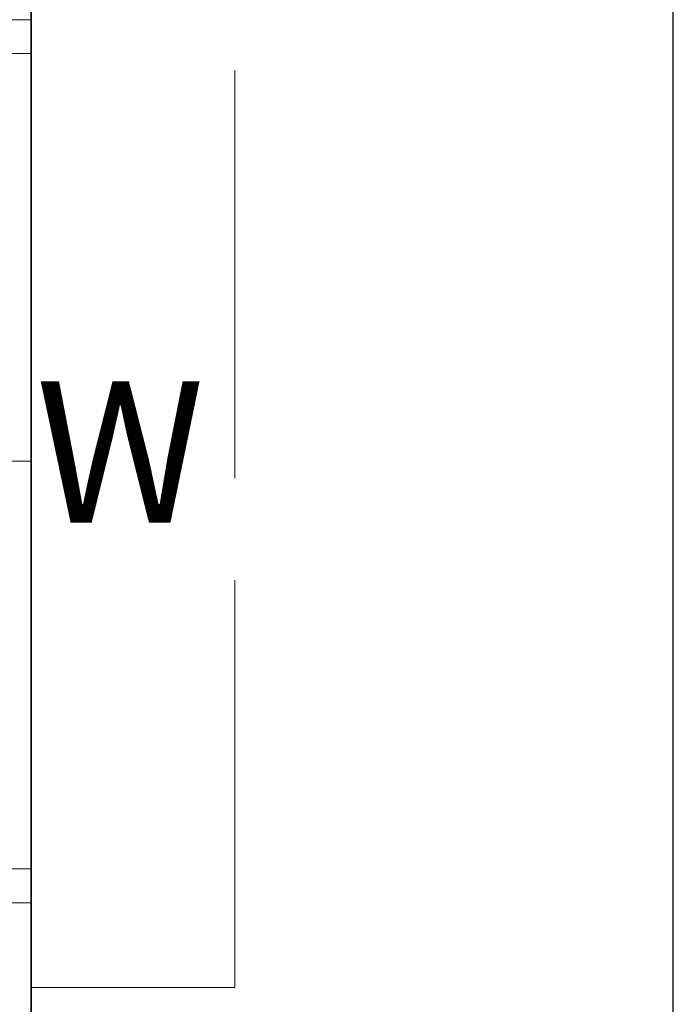
# Model space of a CAD drawing. Units: inches. Extents: x -128 to 854, y -395 to 398.
# Tile 47 of 61: x 313 to 352, y 236 to 294. Entities that reach past the tile are written whole.
import ezdxf

# ---------------------------------------------------------------- set-up
doc = ezdxf.new("R2010")
doc.units = ezdxf.units.IN
doc.header["$MEASUREMENT"] = 0
doc.linetypes.add('ACAD_ISO02W100', pattern=[15, 12, -3])
for name, color, linetype, lineweight in [('A-ANNO-DIMS', 2, 'Continuous', 18), ('A-ANNO-TEXT', 2, 'Continuous', 18), ('A-GLAZ', 220, 'Continuous', 18), ('A-GLAZ-OVHD', 220, 'ACAD_ISO02W100', 13), ('A-WALL', 4, 'Continuous', 35)]:
    doc.layers.add(name, color=color, linetype=linetype, lineweight=lineweight)
doc.styles.get("Standard").update_dxf_attribs({"font": 'arial.ttf'})
doc.dimstyles.get("Standard").update_dxf_attribs({"dimtxt": 0.18, "dimasz": 0.18, "dimexe": 0.18, "dimexo": 0.0625, "dimgap": 0.09, "dimtad": 0, "dimtih": 1, "dimtoh": 1, "dimdec": 1, "dimzin": 0, "dimdsep": 46, "dimlunit": 4, "dimtxsty": 'Standard', "dimcen": 0.09, "dimclrd": 1, "dimclre": 2, "dimclrt": 6, "dimadec": 0, "dimazin": 0, "dimtfac": 1, "dimtdec": 1, "dimtofl": 0, "dimtmove": 0, "dimatfit": 3, "dimfxl": 1, "dimtfill": 2, "dimtfillclr": 3, "dimtolj": 1, "dimtzin": 0, "dimarcsym": 0})

# ---------------------------------------------------------------- blocks, each defined once
blk = doc.blocks.new('WIN-48IN')
for p, q in [((9, 52), (0, 52)), ((9, 50), (0, 50)), ((3.5, 50), (3.5, 2)), ((5.5, 50), (5.5, 2)), ((9, 26), (0, 26)), ((9, 2), (0, 2)), ((9, 0), (0, 0))]:
    blk.add_line(p, q)
blk = doc.blocks.new('SHADE-48IN')
at = {"ltscale": 2}
for p, q in [((0, 0), (0, 62)), ((12, 57), (12, 62)), ((12, 5), (12, 0)), ((12, 0), (0, 0))]:
    blk.add_line(p, q, dxfattribs=at)
blk = doc.blocks.new('*D98')
at = {"layer": 'A-ANNO-DIMS', "color": 2, "lineweight": -2, "transparency": 16777216}
for p, q in [((313.935, 348.741), (351.853, 348.741)), ((313.935, -89.259), (351.853, -89.259))]:
    blk.add_line(p, q, dxfattribs=at)
at = {"layer": 'A-ANNO-DIMS', "color": 1, "lineweight": -2, "transparency": 16777216}
for p, q in [((351.673, 348.561), (351.673, 129.923)), ((351.673, -89.079), (351.673, 129.559))]:
    blk.add_line(p, q, dxfattribs=at)
at = {"layer": 'A-ANNO-DIMS', "color": 1, "transparency": 16777216}
for points in [[(351.643, 348.561), (351.703, 348.561), (351.673, 348.741)], [(351.643, -89.079), (351.703, -89.079), (351.673, -89.259)]]:
    blk.add_solid(points, dxfattribs=at)
at = {"layer": 'Defpoints', "color": 0, "transparency": 16777216}
for p in [(313.873, 348.741), (351.673, 348.741), (313.873, -89.259)]:
    blk.add_point(p, dxfattribs=at)
at = {"layer": 'A-ANNO-DIMS', "color": 6, "transparency": 16777216, "insert": (351.673, 129.741), "char_height": 0.18, "attachment_point": 5, "bg_fill": 1, "box_fill_scale": 1.25, "bg_fill_color": 3, "bg_fill_transparency": 0}
blk.add_mtext('\\A1;36\'-6"', dxfattribs=at)

msp = doc.modelspace()

# ---------------------------------------------------------------- linework, layer by layer
at = {"layer": 'A-WALL'}
msp.add_line((313.873, 348.741), (313.873, -89.259), dxfattribs=at)

# ---------------------------------------------------------------- block references
at = {"layer": 'A-GLAZ'}
msp.add_blockref('WIN-48IN', (304.873, 241.741), dxfattribs=at)
at = {"layer": 'A-GLAZ-OVHD', "extrusion": (0, 0, -1), "zscale": -1}
msp.add_blockref('SHADE-48IN', (-325.873, 236.741), dxfattribs=at)

# ---------------------------------------------------------------- texts
at = {"layer": 'A-ANNO-TEXT'}
msp.add_text('W', height=8.314, dxfattribs=at).set_placement((314.14, 264.131))

# ---------------------------------------------------------------- dimensions: what is measured, and where the dimension line sits
at = {"layer": 'A-ANNO-DIMS'}
dim = msp.add_linear_dim(base=(351.673, 348.741), p1=(313.873, -89.259), p2=(313.873, 348.741), angle=90, dimstyle='Standard', override={"dimdec": 1, "dimlfac": 1, "dimrnd": 0, "dimzin": 1, "dimdsep": 46, "dimlunit": 4, "dimfrac": 2}, dxfattribs=at)
dim.commit()
dim.dimension.update_dxf_attribs({"geometry": '*D98', "text_midpoint": (351.673, 129.741)})

doc.saveas('drawing.dxf')
